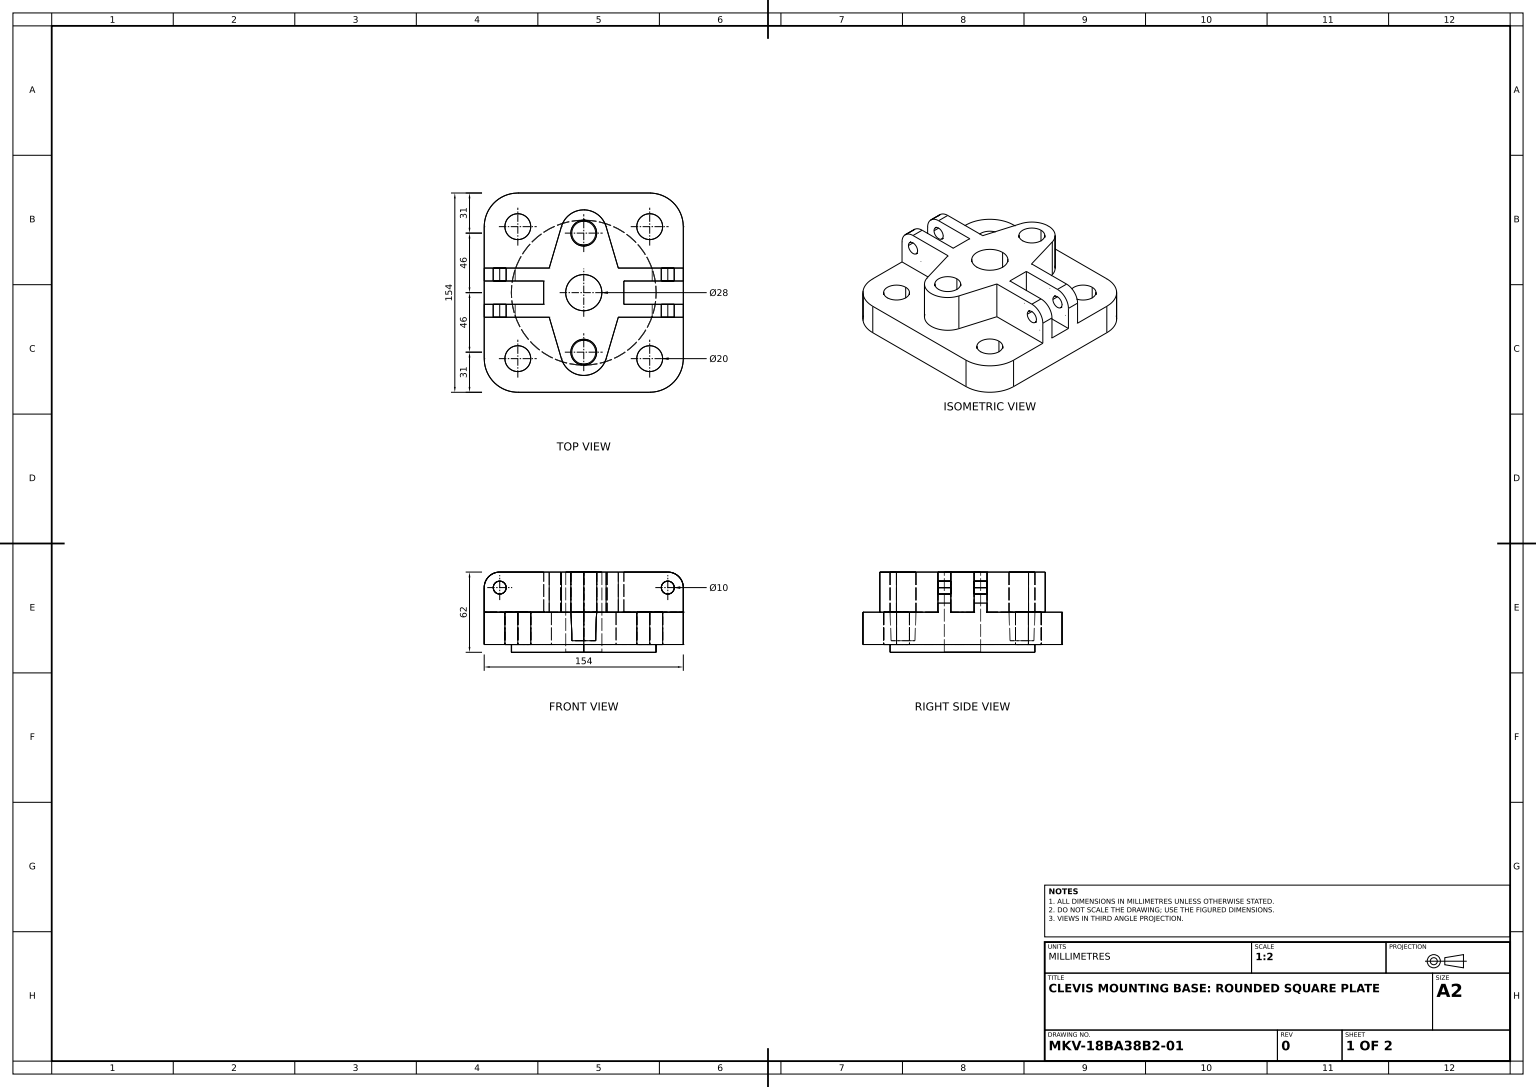
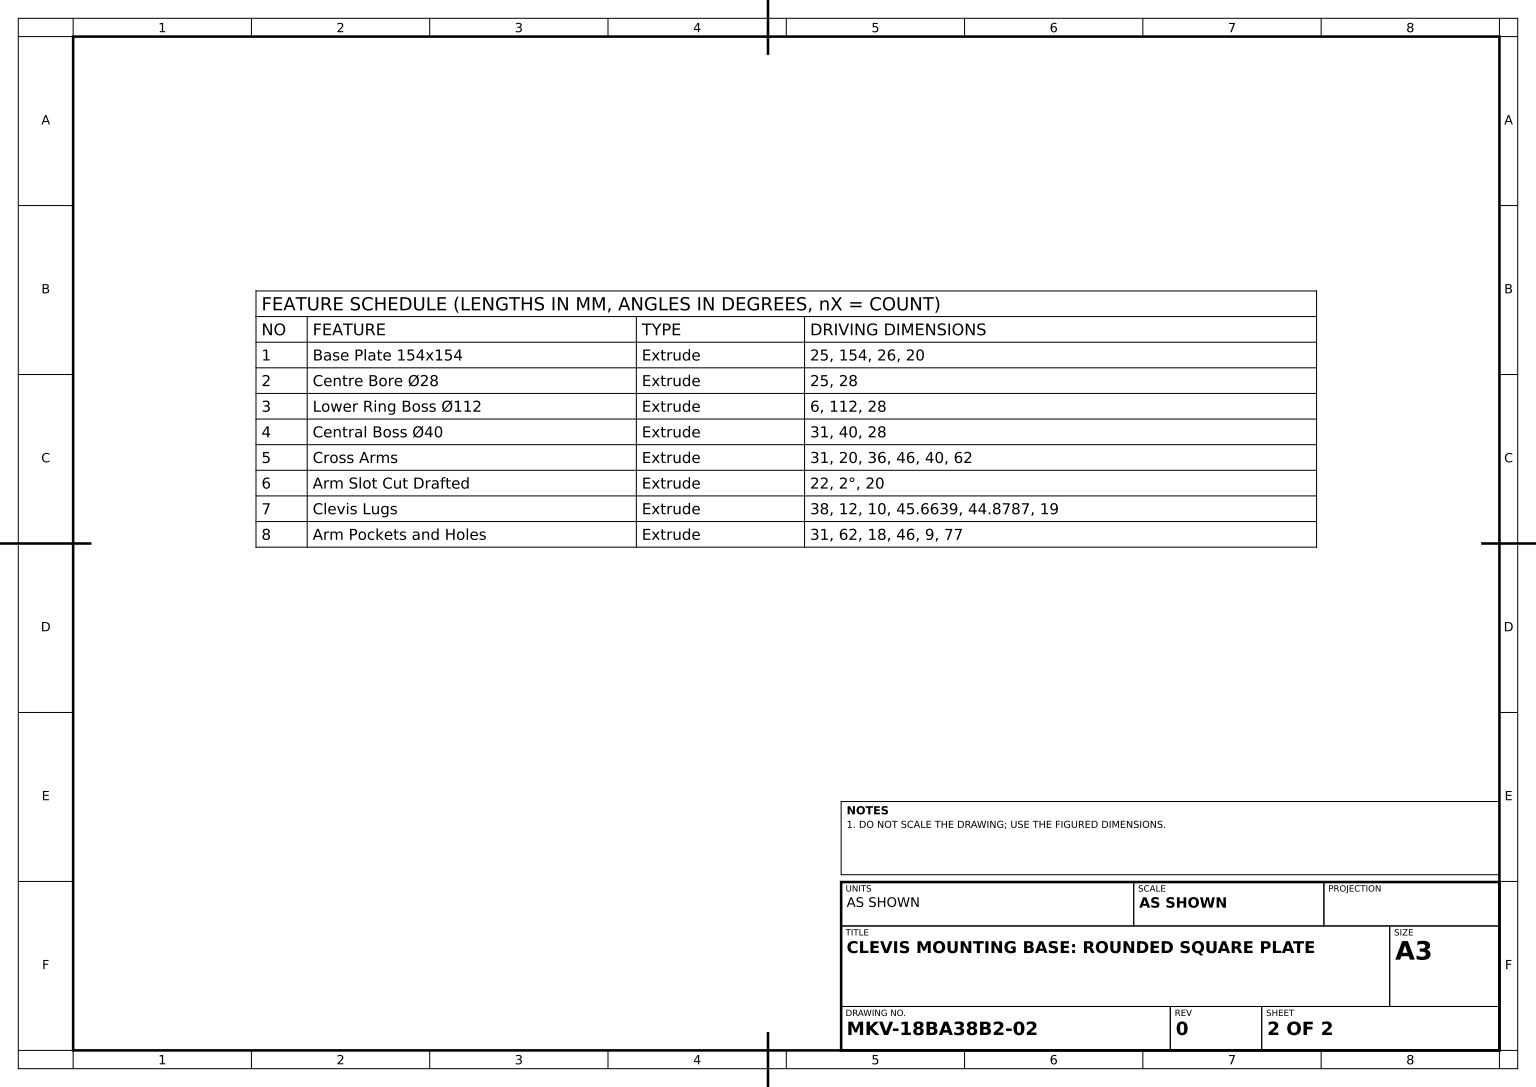
SolidWorks part; units mm, degrees
material "Plain Carbon Steel"
ref_plane "Front Plane" through (0, 0, 0) normal (0, 0, 1) x (1, 0, 0)
ref_plane "Top Plane" through (0, 0, 0) normal (0, 1, 0) x (1, 0, 0)
ref_plane "Right Plane" through (0, 0, 0) normal (1, 0, 0) x (0, 0, -1)
sketch "Base Plate Sketch" plane through (0, 0, 0) normal (0, 1, 0) x (1, 0, 0)
  line L1 (-51, 77) -> (51, 77)
  line L2 (-77, 51) -> (-77, -51)
  line L3 (-51, -77) -> (51, -77)
  line L4 (77, 51) -> (77, -51)
  line L5 (-77, 77) -> (77, -77) construction
  line L6 (-77, -77) -> (77, 77) construction
  arc A0 (51, -77) -> (77, -51) centre (51, -51) ccw
  arc A1 (-77, -51) -> (-51, -77) centre (-51, -51) ccw
  arc A2 (51, 77) -> (77, 51) centre (51, 51) cw
  arc A3 (-51, 77) -> (-77, 51) centre (-51, 51) ccw
  circle A4 centre (-51, 51) radius 10
  circle A5 centre (51, 51) radius 10
  circle A6 centre (51, -51) radius 10
  circle A7 centre (-51, -51) radius 10
  point P0 (0, 0)
  dimension "D2" = 26
  dimension "D3" = 20
  dimension "D4" = 20
  dimension "D5" = 20
  dimension "D6" = 20
  dimension "D1" = 154
extrude "Base Plate 154x154" add sketch "Base Plate Sketch" along normal blind 25
sketch "Centre Bore Sketch" plane through (0, 25, 0) normal (0, 1, 0) x (1, 0, 0)
  circle A0 centre (0, 0) radius 14
  dimension "D1" = 28
extrude "Centre Bore Ø28" cut sketch "Centre Bore Sketch" against normal blind 25
sketch "Lower Ring Boss Sketch" plane through (0, 0, 0) normal (0, -1, 0) x (1, 0, 0)
  circle A0 centre (0, 0) radius 14
  circle A1 centre (0, 0) radius 56
  dimension "D1" = 112
  dimension "D2" = 28
extrude "Lower Ring Boss Ø112" add sketch "Lower Ring Boss Sketch" along normal blind 6
sketch "Central Boss Sketch" plane through (0, 25, 0) normal (0, 1, 0) x (1, 0, 0)
  circle A0 centre (0, 0) radius 14
  circle A1 centre (0, 0) radius 20
  dimension "D1" = 40
  dimension "D2" = 28
extrude "Central Boss Ø40" add sketch "Central Boss Sketch" along normal blind 31
sketch "Cross Arms Sketch" plane through (0, 25, 0) normal (0, 1, 0) x (1, 0, 0)
  line L0 (51, 77) -> (-51, 77) construction
  line L1 (-51, -77) -> (51, -77) construction
  line L4 (-29.7363, 8.7609) -> (-17.2662, 51.087)
  line L5 (29.7363, 8.7609) -> (17.2662, 51.087)
  line L6 (-29.7363, -8.7609) -> (-17.2662, -51.087)
  line L7 (17.2662, -51.087) -> (29.7363, -8.7609)
  arc A0 (17.2662, 51.087) -> (-17.2662, 51.087) centre (0, 46) ccw
  circle A1 centre (0, 46) radius 10
  circle A2 centre (0, -46) radius 10
  arc A3 (-17.2662, -51.087) -> (17.2662, -51.087) centre (0, -46) ccw
  arc A4 (-29.7363, 8.7609) -> (-29.7363, -8.7609) centre (0, 0) ccw
  circle A5 centre (0, 0) radius 20
  arc A6 (29.7363, -8.7609) -> (29.7363, 8.7609) centre (0, 0) ccw
  dimension "D1" = 20
  dimension "D2" = 36
  dimension "D7" = 40
  dimension "D8" = 62
  dimension "D9" = 36
  dimension "D10" = 20
  dimension "D3" = 46
  dimension "D4" = 46
  dimension "D5" = 31
  dimension "D6" = 31
extrude "Cross Arms" add sketch "Cross Arms Sketch" along normal blind 31
sketch "Arm Slot Sketch" plane through (0, 25, 0) normal (0, 1, 0) x (1, 0, 0)
  circle A0 centre (0, 46) radius 10
  circle A1 centre (0, -46) radius 10
  dimension "D1" = 20
  dimension "D2" = 20
extrude "Arm Slot Cut Drafted" cut sketch "Arm Slot Sketch" against normal blind 22 draft 2
ref_plane "Plane1" through (0, 0, 0) normal (0, 0, 1) x (1, 0, 0)
sketch "Clevis Lugs Sketch" plane through (0, 0, 0) normal (0, 0, 1) x (1, 0, 0)
  line L0 (-19.3361, 56) -> (-65, 56)
  line L1 (-29.7363, 56) -> (-17.2662, 56) construction
  line L2 (-77, 44) -> (-77, 25)
  line L3 (-77, 25) -> (-19.3361, 25)
  line L4 (77, 25) -> (77, 44)
  line L5 (65, 56) -> (20.1213, 56)
  line L6 (17.2662, 56) -> (29.7363, 56) construction
  line L7 (-19.3361, 56) -> (-19.3361, 25)
  line L9 (20.1213, 25) -> (20.1213, 56)
  line L10 (20.1213, 25) -> (77, 25)
  arc A0 (77, 44) -> (65, 56) centre (65, 44) ccw
  arc A1 (-65, 56) -> (-77, 44) centre (-65, 44) ccw
  circle A2 centre (-65, 44) radius 5
  circle A3 centre (65, 44) radius 5
  dimension "D1" = 12
  dimension "D2" = 10
  dimension "D3" = 10
  dimension "D4" = 45.6639
  dimension "D5" = 44.8787
  dimension "D6" = 19
extrude "Clevis Lugs" add sketch "Clevis Lugs Sketch" along normal mid plane 38
sketch "Arm Pockets Sketch" plane through (0, 56, 0) normal (0, 1, 0) x (1, 0, 0)
  line L3 (-77, 9) -> (-77, -9)
  line L5 (-77, -9) -> (-31, -9)
  line L7 (31, -9) -> (77, -9)
  line L8 (-77, 9) -> (-31, 9)
  line L10 (31, 9) -> (77, 9)
  line L11 (77, 9) -> (77, -9)
  line L12 (-31, 0) -> (-31, 9)
  line L13 (-31, -9) -> (-31, 0)
  line L14 (31, 0) -> (31, 9)
  line L15 (31, -9) -> (31, 0)
  circle A0 centre (0, 0) radius 31
  point P3 (77, 0)
  line M11 (65, -19) -> (65, 19)
  line M17 (-65, 19) -> (-65, -19)
  dimension "D1" = 62
  dimension "D2" = 18
  dimension "D3" = 46
  dimension "D4" = 9
  dimension "D5" = 77
  dimension "D6" = 9
  dimension "D7" = 77
  dimension "D8" = 9
  dimension "D9" = 18
  dimension "D10" = 9
  dimension "D11" = 9
extrude "Arm Pockets and Holes" cut sketch "Arm Pockets Sketch" against normal blind 31 contours L5 L13 L12 L8 M17 | L8 L3 L5 M17 | L15 L7 L10 L14 M11 | L11 L10 L7 M11
